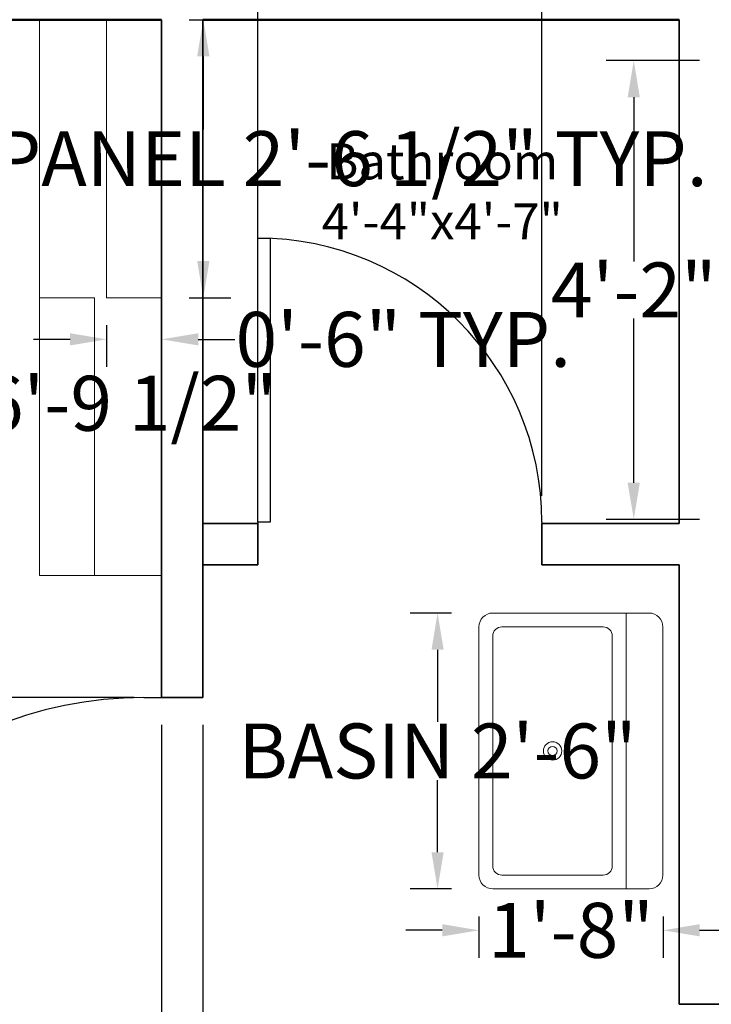
# Model space of a CAD drawing. Units: inches. Extents: x -59 to 502, y -260 to 136.
# Tile 6 of 8: x 151 to 226, y -53 to 55. Entities that reach past the tile are written whole.
import ezdxf

# ---------------------------------------------------------------- set-up
doc = ezdxf.new("R2010")
doc.units = ezdxf.units.IN
doc.header["$MEASUREMENT"] = 0
for name, color, linetype, lineweight in [('A-ANNO-DIMS', 2, 'Continuous', 18), ('A-AREA-IDEN', 7, 'Continuous', 25), ('Closet', 63, 'Continuous', 18), ('Doors', 18, 'Continuous', 25), ('Inner wall', 11, 'Continuous', 35), ('Outer Wall', 10, 'Continuous', 50), ('Sink', 62, 'Continuous', 18)]:
    doc.layers.add(name, color=color, linetype=linetype, lineweight=lineweight)
doc.styles.add('ATTR', font='romans.shx', dxfattribs={"width": 0.8, "height": 1.075})
doc.styles.get("Standard").update_dxf_attribs({"font": 'arial.ttf'})
doc.dimstyles.get("Standard").update_dxf_attribs({"dimtxt": 6, "dimasz": 4, "dimexe": 3, "dimexo": 3, "dimgap": 0.09, "dimtad": 0, "dimtih": 1, "dimtoh": 1, "dimdec": 1, "dimzin": 0, "dimdsep": 46, "dimlunit": 3, "dimtxsty": 'Standard', "dimcen": 0.09, "dimadec": 0, "dimazin": 0, "dimtfac": 1, "dimtdec": 1, "dimtofl": 0, "dimtmove": 0, "dimatfit": 3, "dimfxl": 1, "dimtolj": 1, "dimtzin": 0, "dimarcsym": 0})

# ---------------------------------------------------------------- blocks, each defined once
blk = doc.blocks.new('*U11')
for p, q in [((-40, 0), (-40, 6)), ((0, 0), (0, 6))]:
    blk.add_line(p, q)
blk.add_lwpolyline([(0, 0), (0, -40), (-1.75, -40), (-1.75, 0)], close=True)
blk.add_arc((0, 0), 40, 180, 270)
blk = doc.blocks.new('*U15')
for p, q in [((0, 0), (0, -6)), ((40, 0), (40, -6))]:
    blk.add_line(p, q)
blk.add_lwpolyline([(0, 0), (0, 40), (1.75, 40), (1.75, 0)], close=True)
blk.add_arc((0, 0), 40, 0, 90)
blk = doc.blocks.new("30'' Sink Single PV")
blk.add_line((-15, -3.999996), (15, -3.999996))
for points in [[(-13.5, 0), (13.5, 0)], [(-15, -18.499996), (-15, -1.5)], [(15, -1.5), (15, -18.499996)], [(-12.5, -5.499996), (12.5, -5.499996)], [(-13.5, -17.499996), (-13.5, -6.499996)], [(13.5, -6.499996), (13.5, -17.499996)], [(12.5, -18.499996), (-12.5, -18.499996)], [(13.5, -19.999996), (-13.5, -19.999996)]]:
    blk.add_lwpolyline(points)
for radius in [1, 0.5]:
    blk.add_circle((0, -11.999996), radius)
for centre, radius, start, end in [((-13.5, -1.5), 1.5, 90, 180), ((13.5, -1.5), 1.5, 0, 90), ((-12.5, -6.499996), 1, 90, 180), ((12.5, -6.499996), 1, 0, 90), ((-12.5, -17.499996), 1, 180, 270), ((12.5, -17.499996), 1, 270, 0), ((-13.5, -18.499996), 1.5, 180, 270), ((13.5, -18.499996), 1.5, 270, 0)]:
    blk.add_arc(centre, radius, start, end)
at = {"style": 'ATTR', "width": 0.8, "flags": 9}
blk.add_attdef('ESTCODE', (0, 0), '', height=0.006, dxfattribs=at)
blk = doc.blocks.new('CLOSET-SLIDING-PANEL')
for q in [(0, 30.35), (6, 0)]:
    blk.add_line((0, 0), q)
blk = doc.blocks.new('*D33')
at = {"layer": 'A-ANNO-DIMS', "color": 0, "lineweight": -2, "transparency": 16777216}
for p, q in [((169.46, 54.92), (174.01, 54.92)), ((171.01, 50.92), (171.01, 42.94)), ((171.01, 28.57), (171.01, 36.55)), ((169.46, 24.57), (174.01, 24.57))]:
    blk.add_line(p, q, dxfattribs=at)
at = {"layer": 'A-ANNO-DIMS', "color": 0, "transparency": 16777216}
for points in [[(170.34, 50.92), (171.68, 50.92), (171.01, 54.92)], [(170.34, 28.57), (171.68, 28.57), (171.01, 24.57)]]:
    blk.add_solid(points, dxfattribs=at)
at = {"layer": 'Defpoints', "color": 0, "transparency": 16777216}
for p in [(166.46, 54.92), (171.01, 54.92), (166.46, 24.57)]:
    blk.add_point(p, dxfattribs=at)
at = {"layer": 'A-ANNO-DIMS', "color": 0, "transparency": 16777216, "insert": (171.01, 39.75), "char_height": 6, "attachment_point": 5}
blk.add_mtext('\\A1;CLOSET PANEL 2\'-6 1/2" TYP.', dxfattribs=at)
blk = doc.blocks.new('*D34')
at = {"layer": 'A-ANNO-DIMS', "color": 0, "lineweight": -2, "transparency": 16777216}
for p, q in [((160.46, 21.57), (160.46, 17.02)), ((166.46, 21.57), (166.46, 17.02)), ((156.46, 20.02), (152.46, 20.02)), ((170.46, 20.02), (174.46, 20.02))]:
    blk.add_line(p, q, dxfattribs=at)
at = {"layer": 'A-ANNO-DIMS', "color": 0, "transparency": 16777216}
for points in [[(156.46, 20.69), (156.46, 19.36), (160.46, 20.02)], [(170.46, 20.69), (170.46, 19.36), (166.46, 20.02)]]:
    blk.add_solid(points, dxfattribs=at)
at = {"layer": 'Defpoints', "color": 0, "transparency": 16777216}
for p in [(160.46, 24.57), (166.46, 24.57), (166.46, 20.02)]:
    blk.add_point(p, dxfattribs=at)
at = {"layer": 'A-ANNO-DIMS', "color": 0, "transparency": 16777216, "insert": (192.84, 20.02), "char_height": 6, "attachment_point": 5}
blk.add_mtext('\\A1;0\'-6" TYP.', dxfattribs=at)
blk = doc.blocks.new('*D35')
at = {"layer": 'A-ANNO-DIMS', "color": 0, "lineweight": -2, "transparency": 16777216}
for p, q in [((184.38, 66.92), (184.38, 70.52)), ((208.38, 66.92), (208.38, 70.52)), ((188.38, 67.52), (204.38, 67.52)), ((208.38, 67.52), (212.38, 67.52))]:
    blk.add_line(p, q, dxfattribs=at)
at = {"layer": 'A-ANNO-DIMS', "color": 0, "transparency": 16777216}
for points in [[(188.38, 68.19), (188.38, 66.86), (184.38, 67.52)], [(204.38, 68.19), (204.38, 66.86), (208.38, 67.52)]]:
    blk.add_solid(points, dxfattribs=at)
at = {"layer": 'Defpoints', "color": 0, "transparency": 16777216}
for p in [(208.38, 67.52), (184.38, 63.92), (208.38, 63.92)]:
    blk.add_point(p, dxfattribs=at)
at = {"layer": 'A-ANNO-DIMS', "color": 0, "transparency": 16777216, "insert": (244.99, 67.52), "char_height": 6, "attachment_point": 5}
blk.add_mtext('\\A1;BATH VENT 2\'-0"', dxfattribs=at)
blk = doc.blocks.new('*D45')
at = {"layer": 'A-ANNO-DIMS', "color": 0, "lineweight": -2, "transparency": 16777216}
for p, q in [((129.95, 53.87), (142.2, 53.87)), ((139.2, 49.87), (139.2, 16.23)), ((139.2, -23.8), (139.2, 9.84)), ((129.95, -27.8), (142.2, -27.8))]:
    blk.add_line(p, q, dxfattribs=at)
at = {"layer": 'A-ANNO-DIMS', "color": 0, "transparency": 16777216}
for points in [[(138.53, 49.87), (139.86, 49.87), (139.2, 53.87)], [(138.53, -23.8), (139.86, -23.8), (139.2, -27.8)]]:
    blk.add_solid(points, dxfattribs=at)
at = {"layer": 'Defpoints', "color": 0, "transparency": 16777216}
for p in [(126.95, 53.87), (139.2, 53.87), (126.95, -27.8)]:
    blk.add_point(p, dxfattribs=at)
at = {"layer": 'A-ANNO-DIMS', "color": 0, "transparency": 16777216, "insert": (139.2, 13.04), "char_height": 6, "attachment_point": 5}
blk.add_mtext('\\A1;BED GROUP 6\'-9 1/2"', dxfattribs=at)
blk = doc.blocks.new('*D48')
at = {"layer": 'A-ANNO-DIMS', "color": 0, "lineweight": -2, "transparency": 16777216}
for p, q in [((225.19, 50.45), (215, 50.45)), ((218, 46.45), (218, 28.51)), ((218, 4.36), (218, 22.31)), ((225.19, 0.36), (215, 0.36))]:
    blk.add_line(p, q, dxfattribs=at)
at = {"layer": 'A-ANNO-DIMS', "color": 0, "transparency": 16777216}
for points in [[(217.33, 46.45), (218.66, 46.45), (218, 50.45)], [(217.33, 4.36), (218.66, 4.36), (218, 0.36)]]:
    blk.add_solid(points, dxfattribs=at)
at = {"layer": 'Defpoints', "color": 0, "transparency": 16777216}
for p in [(218, 50.45), (228.19, 50.45), (228.19, 0.36)]:
    blk.add_point(p, dxfattribs=at)
at = {"layer": 'A-ANNO-DIMS', "color": 0, "transparency": 16777216, "insert": (218, 25.41), "char_height": 6, "attachment_point": 5}
blk.add_mtext('\\A1;4\'-2"', dxfattribs=at)
blk = doc.blocks.new('*D55')
at = {"layer": 'A-ANNO-DIMS', "color": 0, "lineweight": -2, "transparency": 16777216}
for p, q in [((198.1, -9.86), (193.58, -9.86)), ((196.58, -13.86), (196.58, -21.73)), ((196.58, -35.98), (196.58, -28.11)), ((198.1, -39.98), (193.58, -39.98))]:
    blk.add_line(p, q, dxfattribs=at)
at = {"layer": 'A-ANNO-DIMS', "color": 0, "transparency": 16777216}
for points in [[(195.92, -13.86), (197.25, -13.86), (196.58, -9.86)], [(195.92, -35.98), (197.25, -35.98), (196.58, -39.98)]]:
    blk.add_solid(points, dxfattribs=at)
at = {"layer": 'Defpoints', "color": 0, "transparency": 16777216}
for p in [(201.1, -9.86), (196.58, -39.98), (201.1, -39.98)]:
    blk.add_point(p, dxfattribs=at)
at = {"layer": 'A-ANNO-DIMS', "color": 0, "transparency": 16777216, "insert": (196.58, -24.92), "char_height": 6, "attachment_point": 5}
blk.add_mtext('\\A1;BASIN 2\'-6"', dxfattribs=at)
blk = doc.blocks.new('*D56')
at = {"layer": 'A-ANNO-DIMS', "color": 0, "lineweight": -2, "transparency": 16777216}
for p, q in [((201.1, -42.98), (201.1, -47.5)), ((221.19, -42.98), (221.19, -47.5)), ((197.1, -44.5), (193.1, -44.5)), ((225.19, -44.5), (229.19, -44.5))]:
    blk.add_line(p, q, dxfattribs=at)
at = {"layer": 'A-ANNO-DIMS', "color": 0, "transparency": 16777216}
for points in [[(197.1, -43.83), (197.1, -45.16), (201.1, -44.5)], [(225.19, -43.83), (225.19, -45.16), (221.19, -44.5)]]:
    blk.add_solid(points, dxfattribs=at)
at = {"layer": 'Defpoints', "color": 0, "transparency": 16777216}
for p in [(201.1, -39.98), (221.19, -39.98), (221.19, -44.5)]:
    blk.add_point(p, dxfattribs=at)
at = {"layer": 'A-ANNO-DIMS', "color": 0, "transparency": 16777216, "insert": (211.15, -44.5), "char_height": 6, "attachment_point": 5}
blk.add_mtext('\\A1;1\'-8"', dxfattribs=at)
blk = doc.blocks.new('*D68')
at = {"layer": 'A-ANNO-DIMS', "color": 0, "lineweight": -2, "transparency": 16777216}
for p, q in [((163.46, -19.08), (-40.87, -19.08)), ((-37.87, -23.08), (-37.87, -37.42)), ((-37.87, -58.08), (-37.87, -43.73)), ((163.46, -62.08), (-40.87, -62.08))]:
    blk.add_line(p, q, dxfattribs=at)
at = {"layer": 'A-ANNO-DIMS', "color": 0, "transparency": 16777216}
for points in [[(-38.53, -23.08), (-37.2, -23.08), (-37.87, -19.08)], [(-38.53, -58.08), (-37.2, -58.08), (-37.87, -62.08)]]:
    blk.add_solid(points, dxfattribs=at)
at = {"layer": 'Defpoints', "color": 0, "transparency": 16777216}
for p in [(166.46, -19.08), (-37.87, -62.08), (166.46, -62.08)]:
    blk.add_point(p, dxfattribs=at)
at = {"layer": 'A-ANNO-DIMS', "color": 0, "transparency": 16777216, "insert": (-37.87, -40.58), "char_height": 6, "attachment_point": 5}
blk.add_mtext('\\A1;3\'-7"', dxfattribs=at)
blk = doc.blocks.new('*D69')
at = {"layer": 'A-ANNO-DIMS', "color": 0, "lineweight": -2, "transparency": 16777216}
for p, q in [((176.96, 2.92), (176.96, 130.25)), ((207.96, 2.92), (207.96, 130.25)), ((180.96, 127.25), (184.34, 127.25)), ((203.96, 127.25), (200.57, 127.25))]:
    blk.add_line(p, q, dxfattribs=at)
at = {"layer": 'A-ANNO-DIMS', "color": 0, "transparency": 16777216}
for points in [[(180.96, 127.91), (180.96, 126.58), (176.96, 127.25)], [(203.96, 127.91), (203.96, 126.58), (207.96, 127.25)]]:
    blk.add_solid(points, dxfattribs=at)
at = {"layer": 'Defpoints', "color": 0, "transparency": 16777216}
for p in [(207.96, 127.25), (176.96, -0.08), (207.96, -0.08)]:
    blk.add_point(p, dxfattribs=at)
at = {"layer": 'A-ANNO-DIMS', "color": 0, "transparency": 16777216, "insert": (192.46, 127.25), "char_height": 6, "attachment_point": 5}
blk.add_mtext('\\A1;2\'-7"', dxfattribs=at)
blk = doc.blocks.new('*D71')
at = {"layer": 'A-ANNO-DIMS', "color": 0, "lineweight": -2, "transparency": 16777216}
for p, q in [((166.46, -22.08), (166.46, -254.4)), ((170.96, -22.08), (170.96, -254.4)), ((162.46, -251.4), (158.46, -251.4)), ((174.96, -251.4), (178.96, -251.4))]:
    blk.add_line(p, q, dxfattribs=at)
at = {"layer": 'A-ANNO-DIMS', "color": 0, "transparency": 16777216}
for points in [[(162.46, -250.74), (162.46, -252.07), (166.46, -251.4)], [(174.96, -250.74), (174.96, -252.07), (170.96, -251.4)]]:
    blk.add_solid(points, dxfattribs=at)
at = {"layer": 'Defpoints', "color": 0, "transparency": 16777216}
for p in [(166.46, -19.08), (170.96, -19.08), (170.96, -251.4)]:
    blk.add_point(p, dxfattribs=at)
at = {"layer": 'A-ANNO-DIMS', "color": 0, "transparency": 16777216, "insert": (194.01, -251.4), "char_height": 6, "attachment_point": 5}
blk.add_mtext('\\A1;0\'-4 1/2"', dxfattribs=at)

msp = doc.modelspace()

# ---------------------------------------------------------------- linework, layer by layer
at = {"layer": 'Closet'}
msp.add_lwpolyline([(153.12, 54.92), (153.12, -5.77), (166.46, -5.77), (166.46, 54.92)], close=True, dxfattribs=at)
at = {"layer": 'Inner wall'}
for p, q in [((166.46, -19.08), (166.46, 54.92)), ((170.96, -4.58), (170.96, 54.92)), ((222.96, -0.08), (222.96, 54.92)), ((170.96, -0.08), (176.96, -0.08)), ((176.96, -4.58), (176.96, -0.08)), ((207.96, -4.58), (207.96, -0.08)), ((207.96, -0.08), (222.96, -0.08)), ((170.96, -4.58), (176.96, -4.58)), ((170.96, -19.08), (170.96, -4.58)), ((207.96, -4.58), (222.96, -4.58)), ((222.96, -52.58), (222.96, -4.58)), ((170.96, -19.08), (166.46, -19.08)), ((222.96, -52.58), (233.46, -52.58))]:
    msp.add_line(p, q, dxfattribs=at)
at = {"layer": 'Outer Wall'}
for p, q in [((34.46, 54.92), (166.46, 54.92)), ((170.96, 54.92), (222.96, 54.92))]:
    msp.add_line(p, q, dxfattribs=at)

# ---------------------------------------------------------------- block references
at = {"layer": 'Closet'}
msp.add_blockref('CLOSET-SLIDING-PANEL', (160.46, 24.57), dxfattribs=at)
at = {"layer": 'Closet', "rotation": 180}
msp.add_blockref('CLOSET-SLIDING-PANEL', (159.12, 24.57), dxfattribs=at)
at = {"layer": 'Doors', "xscale": 0.775, "yscale": 0.775, "zscale": 0.775}
msp.add_blockref('*U15', (176.96, 0.07), dxfattribs=at)
at = {"layer": 'Doors', "xscale": 1.074999999999999, "yscale": 1.074999999999999, "zscale": 1.074999999999999, "rotation": 270}
msp.add_blockref('*U11', (164.51, -62.08), dxfattribs=at)
at = {"layer": 'Sink', "xscale": 1.004024987567037, "yscale": 1.004024987567037, "zscale": 1.004024987567037, "rotation": 270}
msp.add_blockref("30'' Sink Single PV", (221.18, -24.92), dxfattribs=at)

# ---------------------------------------------------------------- texts
at = {"layer": 'A-AREA-IDEN', "insert": (-90.57, 41.41), "char_height": 3.9252, "attachment_point": 1}
msp.add_mtext_dynamic_manual_height_columns('\\pxqc;Bathroom\\P4\'-4"x4\'-7"', width=575.3247, gutter_width=19.63, heights=[0], dxfattribs=at)

# ---------------------------------------------------------------- dimensions: what is measured, and where the dimension line sits
at = {"layer": 'A-ANNO-DIMS'}
for base, p1, p2, picture, middle in [((207.96, 127.25), (176.96, -0.08), (207.96, -0.08), '*D69', (192.46, 127.25)), ((170.96, -251.4), (166.46, -19.08), (170.96, -19.08), '*D71', (194.01, -251.4)), ((221.19, -44.5), (201.1, -39.98), (221.19, -39.98), '*D56', (211.15, -44.5))]:
    dim = msp.add_linear_dim(base=base, p1=p1, p2=p2, dimstyle='Standard', override={"dimdec": 1, "dimlfac": 1, "dimrnd": 0, "dimzin": 1, "dimdsep": 46, "dimlunit": 4, "dimfrac": 2}, dxfattribs=at)
    dim.commit()
    dim.dimension.update_dxf_attribs({"geometry": picture, "text_midpoint": middle})
for base, p1, p2, text, picture, middle in [((208.38, 67.52), (184.38, 63.92), (208.38, 63.92), 'BATH VENT <>', '*D35', (244.99, 67.52)), ((166.46, 20.02), (160.46, 24.57), (166.46, 24.57), '<> TYP.', '*D34', (192.84, 20.02))]:
    dim = msp.add_linear_dim(base=base, p1=p1, p2=p2, text=text, dimstyle='Standard', override={"dimdec": 1, "dimlfac": 1, "dimrnd": 0, "dimzin": 1, "dimdsep": 46, "dimlunit": 4, "dimfrac": 2}, dxfattribs=at)
    dim.commit()
    dim.dimension.update_dxf_attribs({"geometry": picture, "text_midpoint": middle})
for base, p1, p2, angle, text, picture, middle in [((171.0112, 54.9218), (166.4591, 24.5742), (166.4591, 54.9218), 90, 'CLOSET PANEL <> TYP.', '*D33', (171.0112, 39.748)), ((139.2, 53.87), (126.95, -27.8), (126.95, 53.87), 90, 'BED GROUP <>', '*D45', (139.2, 13.04)), ((196.58, -39.98), (201.1, -9.86), (201.1, -39.98), 270, 'BASIN <>', '*D55', (196.58, -24.92))]:
    dim = msp.add_linear_dim(base=base, p1=p1, p2=p2, angle=angle, text=text, dimstyle='Standard', override={"dimdec": 1, "dimlfac": 1, "dimrnd": 0, "dimzin": 1, "dimdsep": 46, "dimlunit": 4, "dimfrac": 2}, dxfattribs=at)
    dim.commit()
    dim.dimension.update_dxf_attribs({"geometry": picture, "text_midpoint": middle})
for base, p1, p2, picture, middle in [((218, 50.45), (228.19, 0.36), (228.19, 50.45), '*D48', (218, 25.41)), ((-37.87, -62.08), (166.46, -19.08), (166.46, -62.08), '*D68', (-37.87, -40.58))]:
    dim = msp.add_linear_dim(base=base, p1=p1, p2=p2, angle=90, dimstyle='Standard', override={"dimdec": 1, "dimlfac": 1, "dimrnd": 0, "dimzin": 1, "dimdsep": 46, "dimlunit": 4, "dimfrac": 2}, dxfattribs=at)
    dim.commit()
    dim.dimension.update_dxf_attribs({"geometry": picture, "text_midpoint": middle})

doc.saveas('drawing.dxf')
